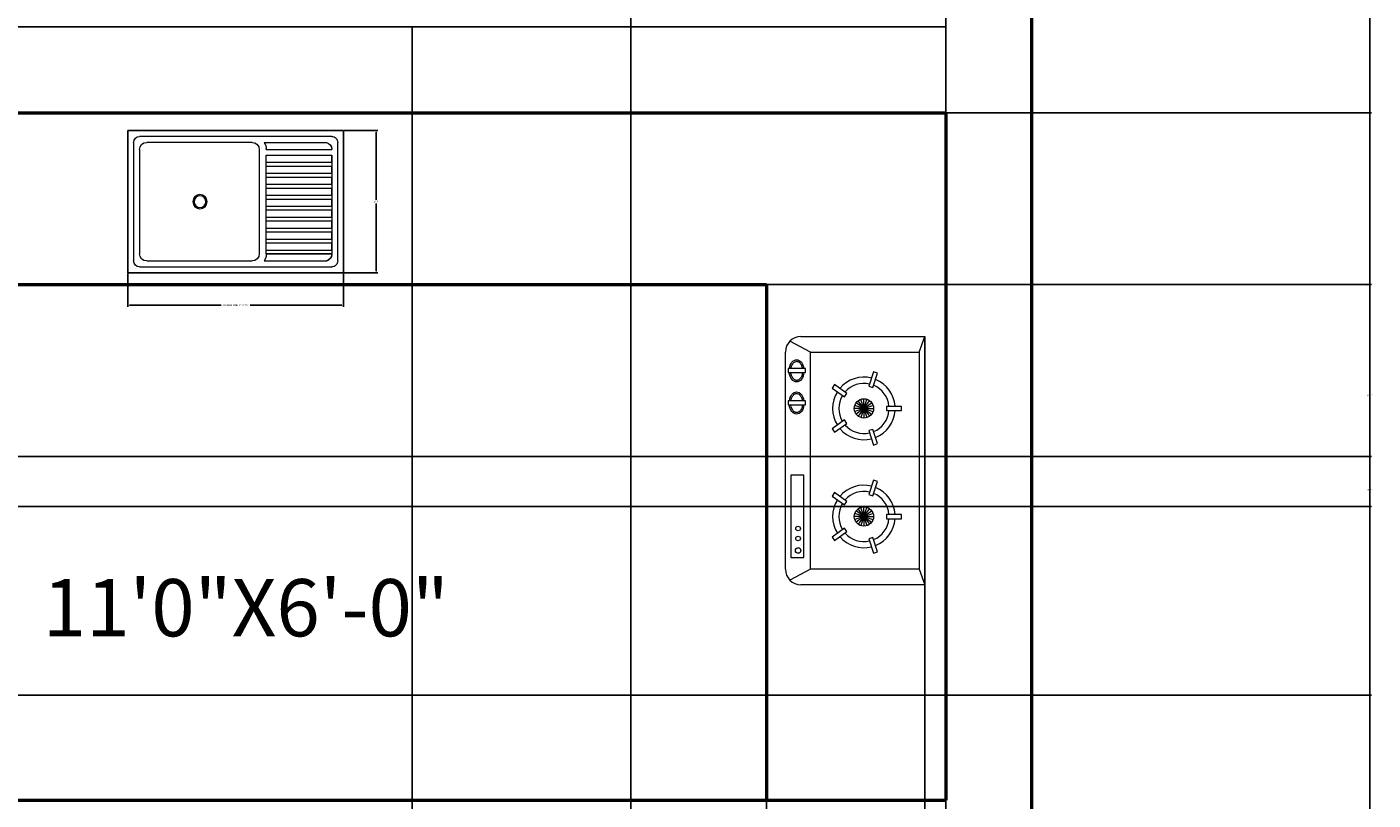
# Model space of a CAD drawing. Units: inches. Extents: x 3 to 576, y -689 to 51.
# Tile 12 of 21: x 435 to 576, y -440 to -359. Entities that reach past the tile are written whole.
import ezdxf

# ---------------------------------------------------------------- set-up
doc = ezdxf.new("R2010")
doc.units = ezdxf.units.IN
doc.header["$MEASUREMENT"] = 0
for name, color, linetype, lineweight in [('A-ANNO-DIMS', 2, 'Continuous', 18), ('A-AREA-IDEN', 7, 'Continuous', 18), ('A-EQPM', 8, 'Continuous', 18), ('A-FLOR-FIXT', 9, 'Continuous', 18), ('A-WALL', 7, 'Continuous', 50)]:
    doc.layers.add(name, color=color, linetype=linetype, lineweight=lineweight)
doc.styles.get("Standard").update_dxf_attribs({"font": 'arial.ttf'})
doc.dimstyles.get("Standard").update_dxf_attribs({"dimtxt": 0.18, "dimasz": 0.18, "dimexe": 0.18, "dimexo": 0.0625, "dimgap": 0.09, "dimtad": 0, "dimtih": 1, "dimtoh": 1, "dimdec": 0, "dimzin": 0, "dimdsep": 46, "dimlunit": 3, "dimtxsty": 'Standard', "dimcen": 0.09, "dimadec": 0, "dimazin": 0, "dimtfac": 1, "dimtdec": 0, "dimtofl": 0, "dimtmove": 0, "dimatfit": 3, "dimfxl": 1, "dimtolj": 1, "dimtzin": 0, "dimarcsym": 0})

# ---------------------------------------------------------------- blocks, each defined once
blk = doc.blocks.new('М12 540х820')
for p, q in [((0, 540), (-820, 540)), ((-820, 540), (-820, 0)), ((-45, 517.5), (-775, 517.5)), ((0, 0), (0, 540)), ((-797.5, 495), (-797.5, 45)), ((-775, 468), (-775, 72)), ((-347.5, 495), (-748, 495)), ((-320.5, 468), (-320.5, 72)), ((-301.7, 495), (-64.8, 495)), ((-293.7, 468), (-293.7, 472.5)), ((-293.7, 468), (-45, 468)), ((-45, 469.5), (-45, 468)), ((-22.5, 45), (-22.5, 495)), ((-293.7, 446.6), (-45, 446.6)), ((-293.7, 419.6), (-293.7, 446.6)), ((-293.7, 419.6), (-45, 419.6)), ((-45, 419.6), (-45, 446.6)), ((-293.7, 405), (-45, 405)), ((-293.7, 378), (-293.7, 405)), ((-293.7, 378), (-45, 378)), ((-293.7, 336.4), (-293.7, 363.4)), ((-293.7, 363.4), (-45, 363.4)), ((-45, 378), (-45, 405)), ((-45, 336.4), (-45, 363.4)), ((-293.7, 336.4), (-45, 336.4)), ((-293.7, 294.7), (-293.7, 321.7)), ((-293.7, 321.7), (-45, 321.7)), ((-45, 294.7), (-45, 321.7)), ((-293.7, 294.7), (-45, 294.7)), ((-293.7, 253.1), (-293.7, 280.1)), ((-293.7, 280.1), (-45, 280.1)), ((-45, 253.1), (-45, 280.1)), ((-293.7, 253.1), (-45, 253.1)), ((-293.7, 211.5), (-293.7, 238.5)), ((-293.7, 238.5), (-45, 238.5)), ((-293.7, 211.5), (-45, 211.5)), ((-45, 211.5), (-45, 238.5)), ((-293.7, 169.9), (-293.7, 196.9)), ((-293.7, 196.9), (-45, 196.9)), ((-293.7, 169.9), (-45, 169.9)), ((-293.7, 128.2), (-293.7, 155.2)), ((-293.7, 155.2), (-45, 155.2)), ((-45, 169.9), (-45, 196.9)), ((-45, 128.2), (-45, 155.2)), ((-293.7, 128.2), (-45, 128.2)), ((-293.7, 113.6), (-45, 113.6)), ((-293.7, 86.6), (-293.7, 113.6)), ((-45, 86.6), (-45, 113.6)), ((-293.7, 86.6), (-45, 86.6)), ((-293.7, 72), (-45, 72)), ((-45, 70.5), (-45, 72)), ((-820, 0), (0, 0)), ((-775, 22.5), (-45, 22.5)), ((-748, 45), (-347.5, 45)), ((-301.7, 45), (-64.8, 45))]:
    blk.add_line(p, q)
at = {"ltscale": 0.06}
for p, q in [((-820, 0), (-820, 540)), ((-820, 540), (0, 540)), ((0, 540), (0, 536.9)), ((0, 536.9), (0, 0)), ((-293.7, 446.6), (-45, 446.6)), ((-293.7, 405), (-293.7, 446.6)), ((-45, 446.6), (-45, 419.6)), ((-45, 419.6), (-45, 378)), ((-293.7, 363.4), (-293.7, 405)), ((-293.7, 321.7), (-293.7, 363.4)), ((-45, 378), (-45, 336.4)), ((-293.7, 280.1), (-293.7, 321.7)), ((-45, 336.4), (-45, 294.7)), ((-293.7, 238.5), (-293.7, 280.1)), ((-45, 294.7), (-45, 253.1)), ((-293.7, 196.9), (-293.7, 238.5)), ((-45, 253.1), (-45, 211.5)), ((-45, 211.5), (-45, 169.9)), ((-293.7, 155.2), (-293.7, 196.9)), ((-293.7, 113.6), (-293.7, 155.2)), ((-45, 169.9), (-45, 128.2)), ((-293.7, 72), (-293.7, 113.6)), ((-45, 128.2), (-45, 86.6)), ((-45, 72), (-293.7, 72)), ((-45, 86.6), (-45, 72)), ((0, 0), (-820, 0))]:
    blk.add_line(p, q, dxfattribs=at)
at = {"extrusion": (0, 0, -1)}
for centre, major_axis, start_param, end_param in [((-775, 495), (-15.9, 15.9), -0.785398, 0.785398), ((-775, 495), (-15.9, 15.9), -0.785398, 0.785398), ((-45, 495), (-15.9, -15.9), 2.356194, 3.926991), ((-45, 495), (-15.9, -15.9), 2.356194, 3.926991), ((-748, 468), (-19.1, -19.1), 0.785398, 2.356194), ((-748, 468), (-19.1, -19.1), 0.785398, 2.356194), ((-347.5, 468), (-19.1, 19.1), 0.785398, 2.356194), ((-347.5, 468), (-19.1, 19.1), 0.785398, 2.356194), ((-343.2, 468), (-35, 35), 1.779263, 2.356194), ((-343.2, 468), (-35, 35), 1.779263, 2.356192), ((-343.2, 468), (-35, 35), 2.356192, 2.356194), ((-72.3, 468.8), (-19.3, 19.3), 1.0328, 2.38382), ((-72.3, 468.8), (-19.3, 19.3), 1.0328, 1.064673), ((-72.3, 468.8), (-19.3, 19.3), 1.064673, 2.328569), ((-72.3, 468.8), (-19.3, 19.3), 2.328569, 2.38382), ((-545.5, 270), (-19.1, -19.1), 3.926991, 10.210176), ((-545.5, 270), (-19.1, -19.1), 3.926991, 10.210176), ((-545.5, 270), (-15.9, -15.9), 3.926991, 10.210176), ((-545.5, 270), (-15.9, -15.9), 3.926991, 10.210176), ((-748, 72), (-19.1, 19.1), 3.926991, 5.497787), ((-748, 72), (-19.1, 19.1), 3.926991, 5.497787), ((-347.5, 72), (-19.1, -19.1), 3.926991, 5.497787), ((-347.5, 72), (-19.1, -19.1), 3.926991, 5.497787), ((-343.2, 72), (-35, -35), 3.926991, 4.503922), ((-343.2, 72), (-35, -35), 3.926991, 4.503922), ((-72.3, 71.2), (-19.3, -19.3), 3.899365, 5.250385), ((-72.3, 71.2), (-19.3, -19.3), 3.954617, 5.218512), ((-72.3, 71.2), (-19.3, -19.3), 3.899365, 3.954617), ((-775, 45), (-15.9, -15.9), 5.497787, 7.068583), ((-775, 45), (-15.9, -15.9), 5.497787, 7.068583), ((-72.3, 71.2), (-19.3, -19.3), 5.218512, 5.250385), ((-45, 45), (-15.9, 15.9), 2.356194, 3.926991), ((-45, 45), (-15.9, 15.9), 2.356194, 3.926991)]:
    blk.add_ellipse(centre, major_axis=major_axis, ratio=1, start_param=start_param, end_param=end_param, dxfattribs=at)
blk = doc.blocks.new('*D27')
at = {"layer": 'A-ANNO-DIMS', "color": 0, "lineweight": -2, "transparency": 16777216}
for p, q in [((445.57, -385.13), (445.57, -388.64)), ((468.19, -385.13), (468.19, -388.64)), ((445.75, -388.46), (455.36, -388.46)), ((468.01, -388.46), (458.4, -388.46))]:
    blk.add_line(p, q, dxfattribs=at)
at = {"layer": 'A-ANNO-DIMS', "color": 0, "transparency": 16777216}
for points in [[(445.75, -388.43), (445.75, -388.49), (445.57, -388.46)], [(468.01, -388.43), (468.01, -388.49), (468.19, -388.46)]]:
    blk.add_solid(points, dxfattribs=at)
at = {"layer": 'Defpoints', "color": 0, "transparency": 16777216}
for p in [(445.57, -385.07), (468.19, -385.07), (468.19, -388.46)]:
    blk.add_point(p, dxfattribs=at)
at = {"layer": 'A-ANNO-DIMS', "color": 0, "transparency": 16777216, "insert": (456.88, -388.46), "char_height": 0.18, "attachment_point": 5}
blk.add_mtext('\\A1;KITCHEN SINK 1\'-10 1/2"', dxfattribs=at)
blk = doc.blocks.new('*D28')
at = {"layer": 'A-ANNO-DIMS', "color": 0, "lineweight": -2, "transparency": 16777216}
for p, q in [((468.26, -370.17), (471.77, -370.17)), ((471.59, -370.35), (471.59, -377.44)), ((471.59, -384.89), (471.59, -377.8)), ((468.26, -385.07), (471.77, -385.07))]:
    blk.add_line(p, q, dxfattribs=at)
at = {"layer": 'A-ANNO-DIMS', "color": 0, "transparency": 16777216}
for points in [[(471.56, -370.35), (471.62, -370.35), (471.59, -370.17)], [(471.56, -384.89), (471.62, -384.89), (471.59, -385.07)]]:
    blk.add_solid(points, dxfattribs=at)
at = {"layer": 'Defpoints', "color": 0, "transparency": 16777216}
for p in [(468.19, -370.17), (471.59, -370.17), (468.19, -385.07)]:
    blk.add_point(p, dxfattribs=at)
at = {"layer": 'A-ANNO-DIMS', "color": 0, "transparency": 16777216, "insert": (471.59, -377.62), "char_height": 0.18, "attachment_point": 5}
blk.add_mtext('\\A1;1\'-3"', dxfattribs=at)
blk = doc.blocks.new('*D39')
at = {"layer": 'A-ANNO-DIMS', "color": 0, "lineweight": -2, "transparency": 16777216}
for p, q in [((540.36, 15.69), (575.92, 15.69)), ((575.74, 15.51), (575.74, -318.63)), ((575.74, -653.13), (575.74, -318.99)), ((540.36, -653.31), (575.92, -653.31))]:
    blk.add_line(p, q, dxfattribs=at)
at = {"layer": 'A-ANNO-DIMS', "color": 0, "transparency": 16777216}
for points in [[(575.71, 15.51), (575.77, 15.51), (575.74, 15.69)], [(575.71, -653.13), (575.77, -653.13), (575.74, -653.31)]]:
    blk.add_solid(points, dxfattribs=at)
at = {"layer": 'Defpoints', "color": 0, "transparency": 16777216}
for p in [(540.29, 15.69), (540.29, -653.31), (575.74, -653.31)]:
    blk.add_point(p, dxfattribs=at)
at = {"layer": 'A-ANNO-DIMS', "color": 0, "transparency": 16777216, "insert": (575.74, -318.81), "char_height": 0.18, "attachment_point": 5}
blk.add_mtext('\\A1;55\'-9"', dxfattribs=at)
blk = doc.blocks.new('*D69')
at = {"layer": 'A-ANNO-DIMS', "color": 0, "lineweight": -2, "transparency": 16777216}
for p, q in [((531.23, -263.31), (2.66, -263.31)), ((2.84, -263.49), (2.84, -311.13)), ((2.84, -359.13), (2.84, -311.49)), ((531.23, -359.31), (2.66, -359.31))]:
    blk.add_line(p, q, dxfattribs=at)
at = {"layer": 'A-ANNO-DIMS', "color": 0, "transparency": 16777216}
for points in [[(2.81, -263.49), (2.87, -263.49), (2.84, -263.31)], [(2.81, -359.13), (2.87, -359.13), (2.84, -359.31)]]:
    blk.add_solid(points, dxfattribs=at)
at = {"layer": 'Defpoints', "color": 0, "transparency": 16777216}
for p in [(531.29, -263.31), (2.84, -359.31), (531.29, -359.31)]:
    blk.add_point(p, dxfattribs=at)
at = {"layer": 'A-ANNO-DIMS', "color": 0, "transparency": 16777216, "insert": (2.84, -311.31), "char_height": 0.18, "attachment_point": 5}
blk.add_mtext('\\A1;8\'-0"', dxfattribs=at)
blk = doc.blocks.new('*D70')
at = {"layer": 'A-ANNO-DIMS', "color": 0, "lineweight": -2, "transparency": 16777216}
for p, q in [((531.23, -359.31), (2.66, -359.31)), ((2.84, -359.49), (2.84, -363.63)), ((2.84, -368.13), (2.84, -363.99)), ((531.23, -368.31), (2.66, -368.31))]:
    blk.add_line(p, q, dxfattribs=at)
at = {"layer": 'A-ANNO-DIMS', "color": 0, "transparency": 16777216}
for points in [[(2.81, -359.49), (2.87, -359.49), (2.84, -359.31)], [(2.81, -368.13), (2.87, -368.13), (2.84, -368.31)]]:
    blk.add_solid(points, dxfattribs=at)
at = {"layer": 'Defpoints', "color": 0, "transparency": 16777216}
for p in [(531.29, -359.31), (2.84, -368.31), (531.29, -368.31)]:
    blk.add_point(p, dxfattribs=at)
at = {"layer": 'A-ANNO-DIMS', "color": 0, "transparency": 16777216, "insert": (2.84, -363.81), "char_height": 0.18, "attachment_point": 5}
blk.add_mtext('\\A1;0\'-9"', dxfattribs=at)
blk = doc.blocks.new('*D71')
at = {"layer": 'A-ANNO-DIMS', "color": 0, "lineweight": -2, "transparency": 16777216}
for p, q in [((531.23, -368.31), (2.66, -368.31)), ((2.84, -368.49), (2.84, -404.13)), ((2.84, -440.13), (2.84, -404.49)), ((531.23, -440.31), (2.66, -440.31))]:
    blk.add_line(p, q, dxfattribs=at)
at = {"layer": 'A-ANNO-DIMS', "color": 0, "transparency": 16777216}
for points in [[(2.81, -368.49), (2.87, -368.49), (2.84, -368.31)], [(2.81, -440.13), (2.87, -440.13), (2.84, -440.31)]]:
    blk.add_solid(points, dxfattribs=at)
at = {"layer": 'Defpoints', "color": 0, "transparency": 16777216}
for p in [(531.29, -368.31), (2.84, -440.31), (531.29, -440.31)]:
    blk.add_point(p, dxfattribs=at)
at = {"layer": 'A-ANNO-DIMS', "color": 0, "transparency": 16777216, "insert": (2.84, -404.31), "char_height": 0.18, "attachment_point": 5}
blk.add_mtext('\\A1;6\'-0"', dxfattribs=at)
blk = doc.blocks.new('*D77')
at = {"layer": 'A-ANNO-DIMS', "color": 0, "lineweight": -2, "transparency": 16777216}
for p, q in [((372.29, -263.37), (372.29, -688.94)), ((531.29, -263.37), (531.29, -688.94)), ((372.47, -688.76), (451.4, -688.76)), ((531.11, -688.76), (452.18, -688.76))]:
    blk.add_line(p, q, dxfattribs=at)
at = {"layer": 'A-ANNO-DIMS', "color": 0, "transparency": 16777216}
for points in [[(372.47, -688.73), (372.47, -688.79), (372.29, -688.76)], [(531.11, -688.73), (531.11, -688.79), (531.29, -688.76)]]:
    blk.add_solid(points, dxfattribs=at)
at = {"layer": 'Defpoints', "color": 0, "transparency": 16777216}
for p in [(372.29, -263.31), (531.29, -263.31), (531.29, -688.76)]:
    blk.add_point(p, dxfattribs=at)
at = {"layer": 'A-ANNO-DIMS', "color": 0, "transparency": 16777216, "insert": (451.79, -688.76), "char_height": 0.18, "attachment_point": 5}
blk.add_mtext('\\A1;13\'-3"', dxfattribs=at)
blk = doc.blocks.new('*D82')
at = {"layer": 'A-ANNO-DIMS', "color": 0, "lineweight": -2, "transparency": 16777216}
for p, q in [((395.37, -359.37), (395.37, -688.94)), ((475.37, -359.37), (475.37, -688.94)), ((395.55, -688.76), (435.04, -688.76)), ((475.19, -688.76), (435.7, -688.76))]:
    blk.add_line(p, q, dxfattribs=at)
at = {"layer": 'A-ANNO-DIMS', "color": 0, "transparency": 16777216}
for points in [[(395.55, -688.73), (395.55, -688.79), (395.37, -688.76)], [(475.19, -688.73), (475.19, -688.79), (475.37, -688.76)]]:
    blk.add_solid(points, dxfattribs=at)
at = {"layer": 'Defpoints', "color": 0, "transparency": 16777216}
for p in [(395.37, -359.31), (475.37, -359.31), (475.37, -688.76)]:
    blk.add_point(p, dxfattribs=at)
at = {"layer": 'A-ANNO-DIMS', "color": 0, "transparency": 16777216, "insert": (435.37, -688.76), "char_height": 0.18, "attachment_point": 5}
blk.add_mtext('\\A1;6\'-8"', dxfattribs=at)
blk = doc.blocks.new('*D83')
at = {"layer": 'A-ANNO-DIMS', "color": 0, "lineweight": -2, "transparency": 16777216}
for p, q in [((475.37, -359.37), (475.37, -688.94)), ((531.29, -359.37), (531.29, -688.94)), ((475.55, -688.76), (503, -688.76)), ((531.11, -688.76), (503.66, -688.76))]:
    blk.add_line(p, q, dxfattribs=at)
at = {"layer": 'A-ANNO-DIMS', "color": 0, "transparency": 16777216}
for points in [[(475.55, -688.73), (475.55, -688.79), (475.37, -688.76)], [(531.11, -688.73), (531.11, -688.79), (531.29, -688.76)]]:
    blk.add_solid(points, dxfattribs=at)
at = {"layer": 'Defpoints', "color": 0, "transparency": 16777216}
for p in [(475.37, -359.31), (531.29, -359.31), (531.29, -688.76)]:
    blk.add_point(p, dxfattribs=at)
at = {"layer": 'A-ANNO-DIMS', "color": 0, "transparency": 16777216, "insert": (503.33, -688.76), "char_height": 0.18, "attachment_point": 5}
blk.add_mtext('\\A1;4\'-8"', dxfattribs=at)
blk = doc.blocks.new('*D91')
at = {"layer": 'A-ANNO-DIMS', "color": 0, "lineweight": -2, "transparency": 16777216}
for p, q in [((181.1, -386.31), (575.92, -386.31)), ((575.74, -386.49), (575.74, -397.75)), ((575.74, -409.38), (575.74, -398.11)), ((181.1, -409.56), (575.92, -409.56))]:
    blk.add_line(p, q, dxfattribs=at)
at = {"layer": 'A-ANNO-DIMS', "color": 0, "transparency": 16777216}
for points in [[(575.71, -386.49), (575.77, -386.49), (575.74, -386.31)], [(575.71, -409.38), (575.77, -409.38), (575.74, -409.56)]]:
    blk.add_solid(points, dxfattribs=at)
at = {"layer": 'Defpoints', "color": 0, "transparency": 16777216}
for p in [(181.04, -386.31), (181.04, -409.56), (575.74, -409.56)]:
    blk.add_point(p, dxfattribs=at)
at = {"layer": 'A-ANNO-DIMS', "color": 0, "transparency": 16777216, "insert": (575.74, -397.93), "char_height": 0.18, "attachment_point": 5}
blk.add_mtext('\\A1;1\'-11"', dxfattribs=at)
blk = doc.blocks.new('*D103')
at = {"layer": 'A-ANNO-DIMS', "color": 0, "lineweight": -2, "transparency": 16777216}
for p, q in [((498.29, -50.37), (498.29, -688.94)), ((531.29, -50.37), (531.29, -688.94)), ((498.47, -688.76), (514.46, -688.76)), ((531.11, -688.76), (515.12, -688.76))]:
    blk.add_line(p, q, dxfattribs=at)
at = {"layer": 'A-ANNO-DIMS', "color": 0, "transparency": 16777216}
for points in [[(498.47, -688.73), (498.47, -688.79), (498.29, -688.76)], [(531.11, -688.73), (531.11, -688.79), (531.29, -688.76)]]:
    blk.add_solid(points, dxfattribs=at)
at = {"layer": 'Defpoints', "color": 0, "transparency": 16777216}
for p in [(498.29, -50.31), (531.29, -50.31), (531.29, -688.76)]:
    blk.add_point(p, dxfattribs=at)
at = {"layer": 'A-ANNO-DIMS', "color": 0, "transparency": 16777216, "insert": (514.79, -688.76), "char_height": 0.18, "attachment_point": 5}
blk.add_mtext('\\A1;2\'-9"', dxfattribs=at)
blk = doc.blocks.new('*D106')
at = {"layer": 'A-ANNO-DIMS', "color": 0, "lineweight": -2, "transparency": 16777216}
for p, q in [((111.36, -386.31), (575.92, -386.31)), ((575.74, -386.49), (575.74, -407.63)), ((575.74, -429.13), (575.74, -407.99)), ((111.36, -429.31), (575.92, -429.31))]:
    blk.add_line(p, q, dxfattribs=at)
at = {"layer": 'A-ANNO-DIMS', "color": 0, "transparency": 16777216}
for points in [[(575.71, -386.49), (575.77, -386.49), (575.74, -386.31)], [(575.71, -429.13), (575.77, -429.13), (575.74, -429.31)]]:
    blk.add_solid(points, dxfattribs=at)
at = {"layer": 'Defpoints', "color": 0, "transparency": 16777216}
for p in [(111.29, -386.31), (111.29, -429.31), (575.74, -429.31)]:
    blk.add_point(p, dxfattribs=at)
at = {"layer": 'A-ANNO-DIMS', "color": 0, "transparency": 16777216, "insert": (575.74, -407.81), "char_height": 0.18, "attachment_point": 5}
blk.add_mtext('\\A1;3\'-7"', dxfattribs=at)
blk = doc.blocks.new('*D110')
at = {"layer": 'A-ANNO-DIMS', "color": 0, "lineweight": -2, "transparency": 16777216}
for p, q in [((397.08, -368.31), (575.92, -368.31)), ((575.74, -368.49), (575.74, -386.13)), ((575.74, -404.13), (575.74, -386.49)), ((397.08, -404.31), (575.92, -404.31))]:
    blk.add_line(p, q, dxfattribs=at)
at = {"layer": 'A-ANNO-DIMS', "color": 0, "transparency": 16777216}
for points in [[(575.71, -368.49), (575.77, -368.49), (575.74, -368.31)], [(575.71, -404.13), (575.77, -404.13), (575.74, -404.31)]]:
    blk.add_solid(points, dxfattribs=at)
at = {"layer": 'Defpoints', "color": 0, "transparency": 16777216}
for p in [(397.02, -368.31), (397.02, -404.31), (575.74, -404.31)]:
    blk.add_point(p, dxfattribs=at)
at = {"layer": 'A-ANNO-DIMS', "color": 0, "transparency": 16777216, "insert": (575.74, -386.31), "char_height": 0.18, "attachment_point": 5}
blk.add_mtext('\\A1;3\'-0"', dxfattribs=at)
blk = doc.blocks.new('*D125')
at = {"layer": 'A-ANNO-DIMS', "color": 0, "lineweight": -2, "transparency": 16777216}
for p, q in [((531.23, -368.31), (2.66, -368.31)), ((2.84, -368.49), (2.84, -377.13)), ((2.84, -386.13), (2.84, -377.49)), ((512.45, -386.31), (2.66, -386.31))]:
    blk.add_line(p, q, dxfattribs=at)
at = {"layer": 'A-ANNO-DIMS', "color": 0, "transparency": 16777216}
for points in [[(2.81, -368.49), (2.87, -368.49), (2.84, -368.31)], [(2.81, -386.13), (2.87, -386.13), (2.84, -386.31)]]:
    blk.add_solid(points, dxfattribs=at)
at = {"layer": 'Defpoints', "color": 0, "transparency": 16777216}
for p in [(531.29, -368.31), (2.84, -386.31), (512.51, -386.31)]:
    blk.add_point(p, dxfattribs=at)
at = {"layer": 'A-ANNO-DIMS', "color": 0, "transparency": 16777216, "insert": (2.84, -377.31), "char_height": 0.18, "attachment_point": 5}
blk.add_mtext('\\A1;1\'-6"', dxfattribs=at)
blk = doc.blocks.new('*D126')
at = {"layer": 'A-ANNO-DIMS', "color": 0, "lineweight": -2, "transparency": 16777216}
for p, q in [((512.51, -386.37), (512.51, -688.94)), ((529.12, -391.8), (529.12, -688.94)), ((512.69, -688.76), (520.28, -688.76)), ((528.94, -688.76), (521.35, -688.76))]:
    blk.add_line(p, q, dxfattribs=at)
at = {"layer": 'A-ANNO-DIMS', "color": 0, "transparency": 16777216}
for points in [[(512.69, -688.73), (512.69, -688.79), (512.51, -688.76)], [(528.94, -688.73), (528.94, -688.79), (529.12, -688.76)]]:
    blk.add_solid(points, dxfattribs=at)
at = {"layer": 'Defpoints', "color": 0, "transparency": 16777216}
for p in [(512.51, -386.31), (529.12, -391.74), (529.12, -688.76)]:
    blk.add_point(p, dxfattribs=at)
at = {"layer": 'A-ANNO-DIMS', "color": 0, "transparency": 16777216, "insert": (520.82, -688.76), "char_height": 0.18, "attachment_point": 5}
blk.add_mtext('\\A1;1\'-4 1/2"', dxfattribs=at)

msp = doc.modelspace()

# ---------------------------------------------------------------- linework, layer by layer
at = {"layer": 'A-EQPM'}
for p, q in [((517.12, -393.37), (514.97, -392.22)), ((516.12, -391.74), (529.12, -391.74)), ((528.5, -393.37), (529.12, -391.74)), ((529.12, -391.74), (529.12, -417.75)), ((514.49, -416.13), (514.49, -393.37)), ((517.12, -393.37), (528.5, -393.37)), ((517.12, -416.13), (517.12, -393.37)), ((528.5, -393.37), (528.5, -416.13)), ((516.58, -395.11), (514.78, -395.11)), ((514.78, -395.11), (514.78, -395.53)), ((514.78, -395.53), (516.58, -395.53)), ((516.58, -395.53), (516.58, -395.11)), ((523.73, -395.46), (523.24, -396.96)), ((523.66, -397.1), (524.15, -395.59)), ((524.15, -395.59), (523.73, -395.46)), ((519.65, -396.78), (519.39, -397.14)), ((519.39, -397.14), (520.67, -398.07)), ((520.93, -397.71), (519.65, -396.78)), ((520.67, -398.07), (520.93, -397.71)), ((523.24, -396.96), (523.66, -397.1)), ((516.58, -398.48), (514.78, -398.48)), ((514.78, -398.48), (514.78, -398.9)), ((514.78, -398.9), (516.58, -398.9)), ((516.58, -398.9), (516.58, -398.48)), ((522.72, -399.28), (521.77, -398.97)), ((522.72, -399.28), (521.91, -398.69)), ((522.72, -399.28), (522.13, -398.47)), ((522.72, -399.28), (522.41, -398.33)), ((522.72, -399.28), (522.72, -398.28)), ((522.72, -399.28), (523.03, -398.33)), ((522.72, -399.28), (523.31, -398.47)), ((522.72, -399.28), (523.53, -398.69)), ((522.72, -399.28), (523.67, -398.97)), ((525.09, -399.06), (525.09, -399.5)), ((526.67, -399.06), (525.09, -399.06)), ((526.67, -399.5), (526.67, -399.06)), ((520.67, -400.49), (519.39, -401.42)), ((520.93, -400.85), (520.67, -400.49)), ((522.72, -399.28), (521.72, -399.28)), ((522.72, -399.28), (521.77, -399.59)), ((522.72, -399.28), (521.91, -399.87)), ((522.72, -399.28), (522.13, -400.09)), ((522.72, -399.28), (522.41, -400.23)), ((522.72, -399.28), (522.72, -400.28)), ((522.72, -399.28), (523.03, -400.23)), ((522.72, -399.28), (523.31, -400.09)), ((522.72, -399.28), (523.53, -399.87)), ((522.72, -399.28), (523.67, -399.59)), ((522.72, -399.28), (523.72, -399.28)), ((525.09, -399.5), (526.67, -399.5)), ((519.39, -401.42), (519.65, -401.78)), ((519.65, -401.78), (520.93, -400.85)), ((523.66, -401.47), (523.24, -401.6)), ((523.24, -401.6), (523.73, -403.11)), ((524.15, -402.97), (523.66, -401.47)), ((523.73, -403.11), (524.15, -402.97)), ((515.05, -406.28), (515.05, -414.88)), ((516.44, -406.28), (515.05, -406.28)), ((516.44, -414.88), (516.44, -406.28)), ((523.73, -406.78), (523.24, -408.28)), ((523.66, -408.42), (524.15, -406.92)), ((524.15, -406.92), (523.73, -406.78)), ((519.65, -408.1), (519.39, -408.46)), ((519.39, -408.46), (520.67, -409.39)), ((520.93, -409.03), (519.65, -408.1)), ((520.67, -409.39), (520.93, -409.03)), ((523.24, -408.28), (523.66, -408.42)), ((522.72, -410.6), (521.77, -410.29)), ((522.72, -410.6), (521.91, -410.02)), ((522.72, -410.6), (522.13, -409.79)), ((522.72, -410.6), (522.41, -409.65)), ((522.72, -410.6), (522.72, -409.6)), ((522.72, -410.6), (523.03, -409.65)), ((522.72, -410.6), (523.31, -409.79)), ((522.72, -410.6), (523.53, -410.02)), ((522.72, -410.6), (523.67, -410.29)), ((525.09, -410.38), (525.09, -410.83)), ((526.67, -410.38), (525.09, -410.38)), ((526.67, -410.83), (526.67, -410.38)), ((520.67, -411.82), (519.39, -412.75)), ((520.93, -412.18), (520.67, -411.82)), ((522.72, -410.6), (521.72, -410.6)), ((522.72, -410.6), (521.77, -410.91)), ((522.72, -410.6), (521.91, -411.19)), ((522.72, -410.6), (522.13, -411.41)), ((522.72, -410.6), (522.41, -411.56)), ((522.72, -410.6), (523.72, -410.6)), ((522.72, -410.6), (523.67, -410.91)), ((522.72, -410.6), (523.53, -411.19)), ((522.72, -410.6), (523.31, -411.41)), ((522.72, -410.6), (523.03, -411.56)), ((522.72, -410.6), (522.72, -411.61)), ((525.09, -410.83), (526.67, -410.83)), ((519.39, -412.75), (519.65, -413.1)), ((519.65, -413.1), (520.93, -412.18)), ((523.66, -412.79), (523.24, -412.93)), ((523.24, -412.93), (523.73, -414.43)), ((524.15, -414.29), (523.66, -412.79)), ((523.73, -414.43), (524.15, -414.29)), ((517.12, -416.13), (514.97, -417.28)), ((515.05, -414.88), (516.44, -414.88)), ((528.5, -416.13), (517.12, -416.13)), ((528.5, -416.13), (529.12, -417.75)), ((529.12, -417.75), (516.12, -417.75))]:
    msp.add_line(p, q, dxfattribs=at)
for centre, radius in [((522.72, -399.28), 1.01), ((522.72, -410.6), 1.01), ((515.82, -411.86), 0.24), ((515.82, -412.91), 0.24), ((515.82, -414.16), 0.288)]:
    msp.add_circle(centre, radius, dxfattribs=at)
for centre, radius, start, end in [((516.12, -393.37), 1.63, 90, 180), ((522.72, -399.28), 3.28, 75.8765, 140.1235), ((522.72, -399.28), 3.28, 3.8765, 68.1235), ((522.72, -399.28), 3.28, 147.8765, 212.1235), ((522.72, -399.28), 2.63, 76.8365, 139.1635), ((522.72, -399.28), 2.63, 4.8365, 67.1635), ((522.72, -399.28), 2.63, 148.8365, 211.1635), ((522.72, -399.28), 2.63, 292.8365, 355.1635), ((522.72, -399.28), 3.28, 291.8765, 356.1235), ((522.72, -399.28), 3.28, 219.8765, 284.1235), ((522.72, -399.28), 2.63, 220.8365, 283.1635), ((522.72, -410.6), 3.28, 75.8765, 140.1235), ((522.72, -410.6), 3.28, 3.8765, 68.1235), ((522.72, -410.6), 3.28, 147.8765, 212.1235), ((522.72, -410.6), 2.63, 76.8365, 139.1635), ((522.72, -410.6), 2.63, 4.8365, 67.1635), ((522.72, -410.6), 2.63, 148.8365, 211.1635), ((522.72, -410.6), 2.63, 292.8365, 355.1635), ((522.72, -410.6), 3.28, 291.8765, 356.1235), ((522.72, -410.6), 3.28, 219.8765, 284.1235), ((522.72, -410.6), 2.63, 220.8365, 283.1635), ((516.12, -416.13), 1.63, 180, 270)]:
    msp.add_arc(centre, radius, start, end, dxfattribs=at)
at = {"layer": 'A-EQPM', "extrusion": (0, 0, -1)}
for centre, major_axis, start_param, end_param in [((515.67, -395.34), (0, -1.16), 1.774361, 4.508825), ((515.67, -395.34), (0, 1.16), 1.73081, 4.552375), ((515.67, -398.71), (0, -1.16), 1.774361, 4.508825), ((515.67, -398.71), (0, 1.16), 1.73081, 4.552375)]:
    msp.add_ellipse(centre, major_axis=major_axis, ratio=0.671641, start_param=start_param, end_param=end_param, dxfattribs=at)
at = {"layer": 'A-EQPM'}
for points, knots in [([(515.07, -395.11), (515.08, -395.05), (515.09, -395), (515.13, -394.87), (515.15, -394.81), (515.21, -394.69), (515.24, -394.63), (515.31, -394.54), (515.35, -394.49), (515.43, -394.43), (515.47, -394.4), (515.55, -394.36), (515.59, -394.35), (515.67, -394.34), (515.7, -394.34), (515.78, -394.36), (515.82, -394.37), (515.9, -394.42), (515.94, -394.44), (516.02, -394.52), (516.06, -394.56), (516.12, -394.66), (516.16, -394.72), (516.21, -394.84), (516.23, -394.91), (516.26, -395.02), (516.27, -395.07), (516.28, -395.11)], [8.079302, 8.079302, 8.079302, 8.079302, 8.245651, 8.245651, 8.463703, 8.463703, 8.681755, 8.681755, 8.899807, 8.899807, 9.117859, 9.117859, 9.33591, 9.33591, 9.553962, 9.553962, 9.772014, 9.772014, 9.990066, 9.990066, 10.208118, 10.208118, 10.426169, 10.426169, 10.644221, 10.644221, 10.770253, 10.770253, 10.770253, 10.770253]), ([(516.28, -395.53), (516.28, -395.57), (516.27, -395.62), (516.25, -395.73), (516.23, -395.8), (516.18, -395.93), (516.15, -395.99), (516.08, -396.1), (516.04, -396.14), (515.97, -396.22), (515.93, -396.26), (515.85, -396.31), (515.81, -396.32), (515.74, -396.34), (515.71, -396.35), (515.67, -396.35), (515.63, -396.35), (515.6, -396.34), (515.52, -396.31), (515.48, -396.29), (515.4, -396.24), (515.36, -396.2), (515.28, -396.12), (515.25, -396.07), (515.19, -395.96), (515.16, -395.9), (515.11, -395.76), (515.09, -395.69), (515.07, -395.59), (515.07, -395.56), (515.07, -395.53)], [4.889299, 4.889299, 4.889299, 4.889299, 5.015191, 5.015191, 5.233243, 5.233243, 5.451295, 5.451295, 5.669347, 5.669347, 5.887399, 5.887399, 6.10545, 6.10545, 6.283185, 6.283185, 6.283185, 6.501237, 6.501237, 6.719289, 6.719289, 6.937341, 6.937341, 7.155392, 7.155392, 7.373444, 7.373444, 7.591496, 7.591496, 7.677072, 7.677072, 7.677072, 7.677072]), ([(515.07, -398.48), (515.08, -398.42), (515.09, -398.37), (515.13, -398.24), (515.15, -398.18), (515.21, -398.05), (515.24, -398), (515.31, -397.9), (515.35, -397.86), (515.43, -397.8), (515.47, -397.77), (515.55, -397.73), (515.59, -397.72), (515.67, -397.71), (515.7, -397.71), (515.78, -397.73), (515.82, -397.74), (515.9, -397.78), (515.94, -397.81), (516.02, -397.88), (516.06, -397.93), (516.12, -398.03), (516.16, -398.09), (516.21, -398.21), (516.23, -398.28), (516.26, -398.39), (516.27, -398.43), (516.28, -398.48)], [8.079302, 8.079302, 8.079302, 8.079302, 8.245651, 8.245651, 8.463703, 8.463703, 8.681755, 8.681755, 8.899807, 8.899807, 9.117859, 9.117859, 9.33591, 9.33591, 9.553962, 9.553962, 9.772014, 9.772014, 9.990066, 9.990066, 10.208118, 10.208118, 10.426169, 10.426169, 10.644221, 10.644221, 10.770253, 10.770253, 10.770253, 10.770253]), ([(516.28, -398.9), (516.28, -398.94), (516.27, -398.98), (516.25, -399.1), (516.23, -399.17), (516.18, -399.3), (516.15, -399.36), (516.08, -399.47), (516.04, -399.51), (515.97, -399.59), (515.93, -399.62), (515.85, -399.67), (515.81, -399.69), (515.74, -399.71), (515.71, -399.71), (515.67, -399.71), (515.63, -399.71), (515.6, -399.71), (515.52, -399.68), (515.48, -399.66), (515.4, -399.61), (515.36, -399.57), (515.28, -399.49), (515.25, -399.44), (515.19, -399.33), (515.16, -399.26), (515.11, -399.13), (515.09, -399.06), (515.07, -398.96), (515.07, -398.93), (515.07, -398.9)], [4.889299, 4.889299, 4.889299, 4.889299, 5.015191, 5.015191, 5.233243, 5.233243, 5.451295, 5.451295, 5.669347, 5.669347, 5.887399, 5.887399, 6.10545, 6.10545, 6.283185, 6.283185, 6.283185, 6.501237, 6.501237, 6.719289, 6.719289, 6.937341, 6.937341, 7.155392, 7.155392, 7.373444, 7.373444, 7.591496, 7.591496, 7.677072, 7.677072, 7.677072, 7.677072])]:
    msp.add_open_spline(points, degree=3, knots=knots, dxfattribs=at)
at = {"layer": 'A-WALL'}
for p, q in [((540.29, 15.69), (540.29, -653.31)), ((397.02, -368.31), (531.29, -368.31)), ((531.29, -368.31), (531.29, -440.31)), ((397.02, -386.31), (512.51, -386.31)), ((512.51, -386.31), (512.51, -440.31)), ((388.02, -440.31), (531.29, -440.31))]:
    msp.add_line(p, q, dxfattribs=at)

# ---------------------------------------------------------------- block references
at = {"layer": 'A-FLOR-FIXT', "xscale": 0.0275962273819375, "yscale": 0.0275962273819375, "zscale": 0.0275962273819375}
msp.add_blockref('М12 540х820', (468.19, -385.07), dxfattribs=at)

# ---------------------------------------------------------------- texts
at = {"layer": 'A-AREA-IDEN', "insert": (436.67, -417.16), "char_height": 6, "attachment_point": 1}
msp.add_mtext_dynamic_manual_height_columns('11\'0"X6\'-0"', width=0.3236, gutter_width=1, heights=[0], dxfattribs=at)

# ---------------------------------------------------------------- dimensions: what is measured, and where the dimension line sits
at = {"layer": 'A-ANNO-DIMS'}
for base, p1, p2, picture, middle in [((575.74, -653.31), (540.29, 15.69), (540.29, -653.31), '*D39', (575.74, -318.81)), ((2.84, -359.31), (531.29, -263.31), (531.29, -359.31), '*D69', (2.84, -311.31)), ((2.84, -368.31), (531.29, -359.31), (531.29, -368.31), '*D70', (2.84, -363.81)), ((2.84, -440.31), (531.29, -368.31), (531.29, -440.31), '*D71', (2.84, -404.31)), ((2.84, -386.31), (531.29, -368.31), (512.51, -386.31), '*D125', (2.84, -377.31)), ((575.74, -404.31), (397.02, -368.31), (397.02, -404.31), '*D110', (575.74, -386.31)), ((471.59, -370.17), (468.19, -385.07), (468.19, -370.17), '*D28', (471.59, -377.62)), ((575.74, -429.31), (111.29, -386.31), (111.29, -429.31), '*D106', (575.74, -407.81)), ((575.744, -409.5571), (181.036, -386.3097), (181.036, -409.5571), '*D91', (575.744, -397.9334))]:
    dim = msp.add_linear_dim(base=base, p1=p1, p2=p2, angle=90, dimstyle='Standard', override={"dimdec": 1, "dimlfac": 1, "dimrnd": 0, "dimzin": 1, "dimdsep": 46, "dimlunit": 4, "dimfrac": 2}, dxfattribs=at)
    dim.commit()
    dim.dimension.update_dxf_attribs({"geometry": picture, "text_midpoint": middle})
for base, p1, p2, picture, middle in [((531.29, -688.76), (498.29, -50.31), (531.29, -50.31), '*D103', (514.79, -688.76)), ((531.29, -688.76), (372.29, -263.31), (531.29, -263.31), '*D77', (451.79, -688.76)), ((475.37, -688.76), (395.37, -359.31), (475.37, -359.31), '*D82', (435.37, -688.76)), ((531.29, -688.76), (475.37, -359.31), (531.29, -359.31), '*D83', (503.33, -688.76)), ((529.12, -688.76), (512.51, -386.31), (529.12, -391.74), '*D126', (520.82, -688.76))]:
    dim = msp.add_linear_dim(base=base, p1=p1, p2=p2, dimstyle='Standard', override={"dimdec": 1, "dimlfac": 1, "dimrnd": 0, "dimzin": 1, "dimdsep": 46, "dimlunit": 4, "dimfrac": 2}, dxfattribs=at)
    dim.commit()
    dim.dimension.update_dxf_attribs({"geometry": picture, "text_midpoint": middle})
dim = msp.add_linear_dim(base=(468.19, -388.46), p1=(445.57, -385.07), p2=(468.19, -385.07), text='KITCHEN SINK <>', dimstyle='Standard', override={"dimdec": 1, "dimlfac": 1, "dimrnd": 0, "dimzin": 1, "dimdsep": 46, "dimlunit": 4, "dimfrac": 2}, dxfattribs=at)
dim.commit()
dim.dimension.update_dxf_attribs({"geometry": '*D27', "text_midpoint": (456.88, -388.46)})

doc.saveas('drawing.dxf')
